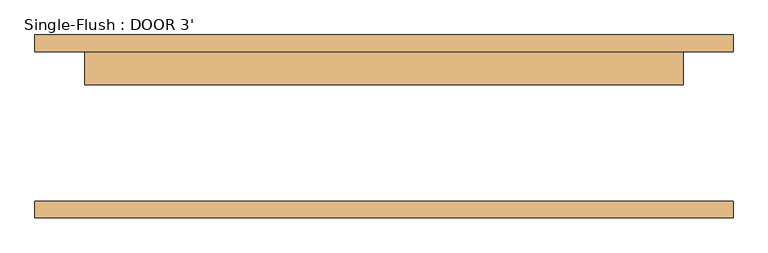
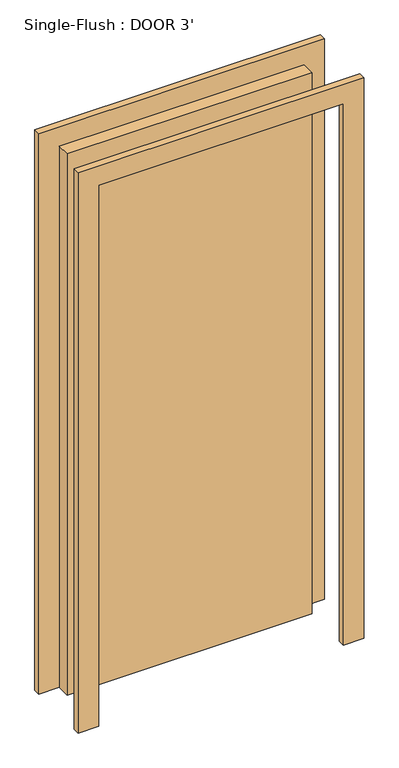
"""IFC4 building model written with IfcOpenShell, lengths in millimetres: door geometry, Single-Flush : DOOR 3'."""

from ifc_helpers import new_model, si_unit, frame, origin, origin_with_axes, place, context, project, spatial, polyline, outline, extrude, source, transform, mapped, element, save


def single_flush_door_3_0ca8825f(model_context):
    return source(origin(), model_context, "Body", "SweptSolid", [
        extrude(outline(polyline([(2209.8, -533.4), (0.0, -533.4), (0.0, -457.2), (2133.6, -457.2), (2133.6, 457.2), (0.0, 457.2), (0.0, 533.4), (2209.8, 533.4), (2209.8, -533.4)])), frame((0.0, 114.3, 0.0), z_axis=(0.0, 1.0, 0.0), x_axis=(0.0, 0.0, 1.0)), (0.0, 0.0, 1.0), 25.4),
        extrude(outline(polyline([(2209.8, 533.4), (2209.8, -533.4), (0.0, -533.4), (0.0, -457.2), (2133.6, -457.2), (2133.6, 457.2), (0.0, 457.2), (0.0, 533.4), (2209.8, 533.4)])), frame((0.0, -139.7, 0.0), z_axis=(0.0, 1.0, 0.0), x_axis=(0.0, 0.0, 1.0)), (0.0, 0.0, 1.0), 25.4),
        extrude(outline(polyline([(457.2, 63.5), (-457.2, 63.5), (-457.2, 114.3), (457.2, 114.3), (457.2, 63.5)])), origin_with_axes(), (0.0, 0.0, 1.0), 2133.6),
    ])


if __name__ == "__main__":
    model = new_model("IFC4")
    model_context = context("Model", 3, world=origin())
    ifc_project = project(units=[si_unit("LENGTHUNIT", "METRE", prefix="MILLI")], contexts=[model_context])
    site = spatial("IfcSite", under=ifc_project)
    building = spatial("IfcBuilding", under=site)
    placement = place(None, origin())
    single_flush_door_3_shape = single_flush_door_3_0ca8825f(model_context)
    element("IfcDoor", 1, ObjectType="Single-Flush : DOOR 3'", at=placement, inside=building, context=model_context, shape_type="MappedRepresentation", body=[
        mapped(single_flush_door_3_shape, transform((0.0, 0.0, 0.0), x_axis=(1.0, 0.0, 0.0), y_axis=(0.0, 1.0, 0.0), z_axis=(0.0, 0.0, 1.0))),
    ])
    save(model, "model.ifc")

# Revit data of these elements
# Type "Single-Flush : DOOR 3'"
#   Type Mark = "9"
#   Construction Type Id = "MDOOR"
#   Assembly Code = "C1020"
#   Analytic Construction = "Metal"
#   Thickness = 0' - 2"
#   Heat Transfer Coefficient (U) = 0.651978 BTU/(h·ft²·°F)
#   Height = 7' - 0"
#   Trim Projection Ext = 0' - 1"
#   Trim Projection Int = 0' - 1"
#   Trim Width = 0' - 3"
#   Width = 3' - 0"
#   Define Thermal Properties by = 1
#   Door Material = Door - Panel
#   Frame Material = Door - Frame
#   Visual Light Transmittance = 0
#   Solar Heat Gain Coefficient = 0
#   Function = (empty or 0)
#   Wall Closure = (empty or 0)
# Element 1 (IfcDoor, "Single-Flush : DOOR 3'")
#   Materials on its faces: "Door - Frame", "Door - Panel"
# Materials
#   "Door - Panel": class "Wood", colour RGB 210 159 95, transparency 0, Cost = 0
#   "Door - Frame": colour RGB 118 70 51, transparency 0, Cost = 0
